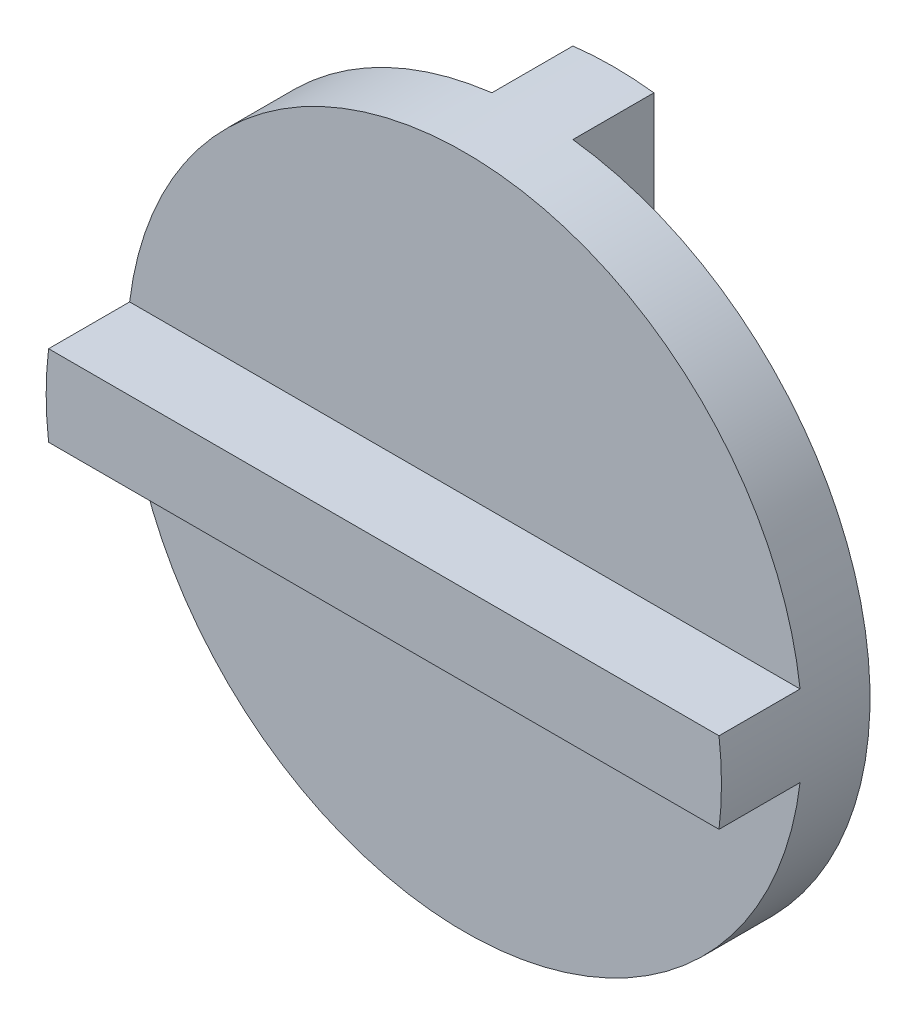
SolidWorks part; units mm, degrees
material "Plain Carbon Steel"
ref_plane "Front Plane" through (0, 0, 0) normal (0, 0, 1) x (1, 0, 0)
ref_plane "Top Plane" through (0, 0, 0) normal (0, 1, 0) x (1, 0, 0)
ref_plane "Right Plane" through (0, 0, 0) normal (1, 0, 0) x (0, 0, -1)
sketch "Disc Profile Ø100" plane through (0, 0, 0) normal (0, 0, 1) x (1, 0, 0)
  circle A0 centre (0, 0) radius 50
  dimension "D1" = 100
extrude "Disc Body" add sketch "Disc Profile Ø100" along normal mid plane 10
sketch "Face Rib 1 Profile" plane through (0, 0, 5) normal (0, 0, 1) x (1, 0, 0)
  line L0 (61.4964, 0) -> (-71.0965, 0) construction
  line L2 (49.6387, -6) -> (-49.6387, -6)
  line L4 (49.6387, 6) -> (-49.6387, 6)
  line L6 (49.6387, -6) -> (-49.6387, 6) construction
  line L7 (49.6387, 6) -> (-49.6387, -6) construction
  circle A0 centre (0, 0) radius 50 construction
  arc A1 (49.6387, -6) -> (49.6387, 6) centre (0, 0) ccw
  arc A2 (-49.6387, 6) -> (-49.6387, -6) centre (0, 0) ccw
  dimension "D1" = 12
extrude "Face Rib 1" add sketch "Face Rib 1 Profile" along normal blind 12
sketch "Face Rib 2 Profile" plane through (0, 0, -5) normal (0, 0, -1) x (-1, 0, 0)
  line L0 (0, -53.3572) -> (0, 53.0789) construction
  line L3 (-6, -49.6387) -> (-6, 49.6387)
  line L5 (6, -49.6387) -> (6, 49.6387)
  line L6 (-6, -49.6387) -> (6, 49.6387) construction
  line L7 (-6, 49.6387) -> (6, -49.6387) construction
  circle A0 centre (0, 0) radius 50 construction
  arc A1 (-6, -49.6387) -> (6, -49.6387) centre (0, 0) ccw
  arc A2 (6, 49.6387) -> (-6, 49.6387) centre (0, 0) ccw
  dimension "D1" = 12
extrude "Face Rib 2" add sketch "Face Rib 2 Profile" along normal blind 12
